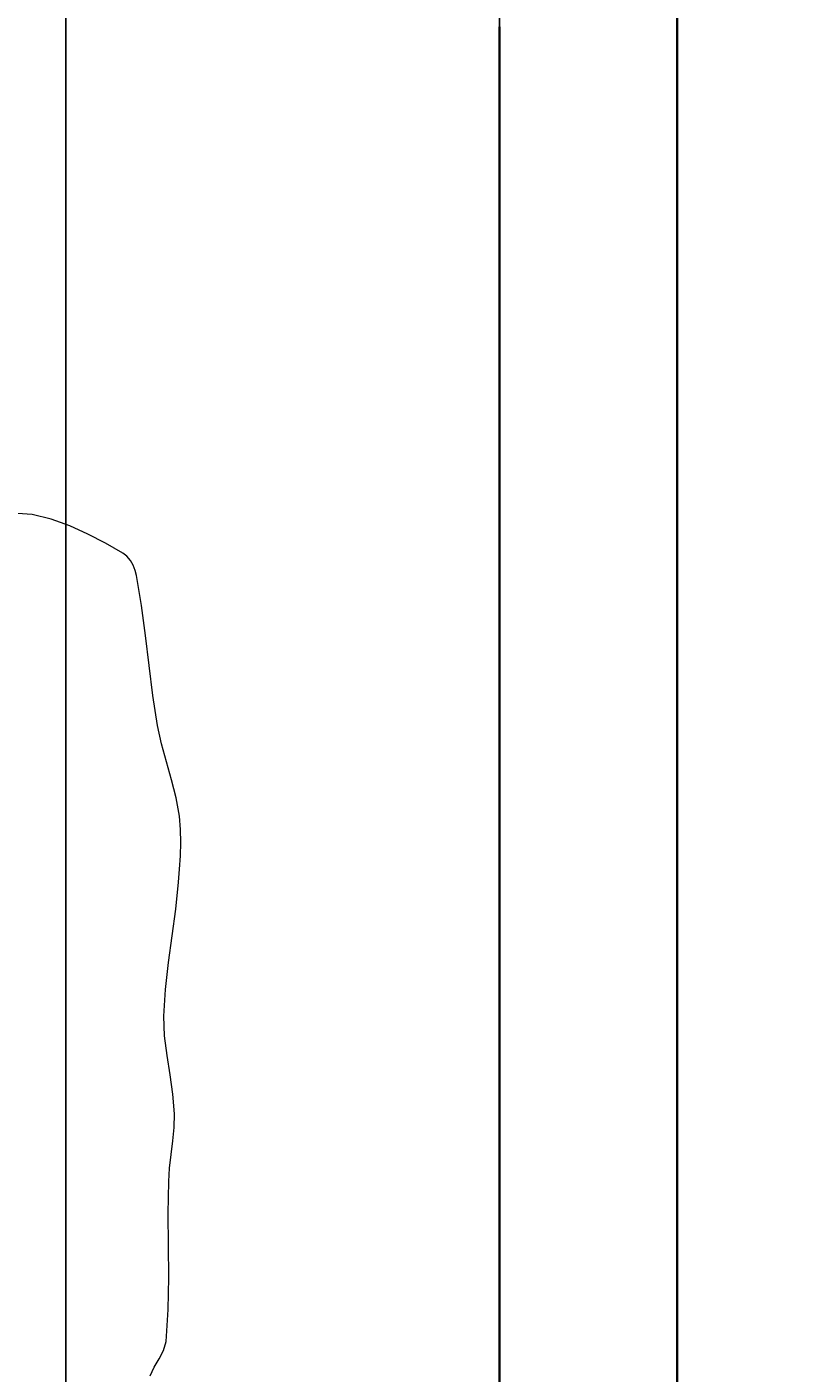
# Model space of a CAD drawing. Units: inches. Extents: x 1770 to 2988, y 1161 to 3221.
# Tile 29 of 44: x 2593 to 2631, y 2300 to 2368. Entities that reach past the tile are written whole.
import ezdxf

# ---------------------------------------------------------------- set-up
doc = ezdxf.new("R2010")
doc.units = ezdxf.units.IN
for name, color, linetype, lineweight in [('A-ANNO-DIMS', 2, 'Continuous', 18), ('A-FURN', 8, 'Continuous', 13), ('A-WALL', 7, 'Continuous', 35)]:
    doc.layers.add(name, color=color, linetype=linetype, lineweight=lineweight)
doc.styles.get("Standard").update_dxf_attribs({"font": 'arial.ttf'})
doc.dimstyles.get("Standard").update_dxf_attribs({"dimtxt": 0.18, "dimasz": 0.18, "dimexe": 0.18, "dimexo": 0.0625, "dimgap": 0.09, "dimtad": 0, "dimtih": 1, "dimtoh": 1, "dimdec": 4, "dimzin": 0, "dimdsep": 46, "dimtxsty": 'Standard', "dimcen": 0.09, "dimadec": 0, "dimazin": 0, "dimtfac": 1, "dimtdec": 4, "dimtofl": 0, "dimtmove": 0, "dimatfit": 3, "dimfxl": 1, "dimtolj": 1, "dimtzin": 0, "dimarcsym": 0})

# ---------------------------------------------------------------- blocks, each defined once
blk = doc.blocks.new('BED-DOUBLE-PLAN')
for p, q in [((67.458, 87.108), (66.715, 87.159)), ((68.424, 86.867), (67.458, 87.108)), ((69.364, 86.53), (68.424, 86.867)), ((70.28, 86.118), (69.364, 86.53)), ((71.172, 85.653), (70.28, 86.118)), ((72.043, 85.157), (71.172, 85.653)), ((72.253, 84.994), (72.043, 85.157)), ((72.425, 84.785), (72.253, 84.994)), ((72.561, 84.542), (72.425, 84.785)), ((72.662, 84.282), (72.561, 84.542)), ((72.731, 84.019), (72.662, 84.282)), ((72.993, 82.51), (72.731, 84.019)), ((73.197, 80.991), (72.993, 82.51)), ((73.377, 79.468), (73.197, 80.991)), ((73.567, 77.947), (73.377, 79.468)), ((73.802, 76.433), (73.567, 77.947)), ((74.003, 75.51), (73.802, 76.433)), ((74.25, 74.596), (74.003, 75.51)), ((74.506, 73.685), (74.25, 74.596)), ((74.736, 72.768), (74.506, 73.685)), ((74.904, 71.84), (74.736, 72.768)), ((74.965, 71.175), (74.904, 71.84)), ((74.978, 70.506), (74.965, 71.175)), ((74.957, 69.836), (74.978, 70.506)), ((74.914, 69.165), (74.957, 69.836)), ((74.862, 68.497), (74.914, 69.165)), ((74.721, 67.139), (74.862, 68.497)), ((74.536, 65.785), (74.721, 67.139)), ((74.348, 64.431), (74.536, 65.785)), ((74.196, 63.075), (74.348, 64.431)), ((74.12, 61.714), (74.196, 63.075)), ((74.159, 60.723), (74.12, 61.714)), ((74.28, 59.737), (74.159, 60.723)), ((74.435, 58.752), (74.28, 59.737)), ((74.575, 57.766), (74.435, 58.752)), ((74.652, 56.776), (74.575, 57.766)), ((74.639, 56.089), (74.652, 56.776)), ((74.578, 55.403), (74.639, 56.089)), ((74.494, 54.718), (74.578, 55.403)), ((74.414, 54.032), (74.494, 54.718)), ((74.365, 53.345), (74.414, 54.032)), ((74.338, 51.727), (74.365, 53.345)), ((74.351, 50.106), (74.338, 51.727)), ((74.364, 48.487), (74.351, 50.106)), ((74.337, 46.869), (74.364, 48.487)), ((74.232, 45.256), (74.337, 46.869)), ((74.11, 44.804), (74.232, 45.256)), ((73.637, 43.953), (73.887, 44.375)), ((73.887, 44.375), (74.11, 44.804)), ((73.435, 43.523), (73.637, 43.953))]:
    blk.add_line(p, q)
blk = doc.blocks.new('*D61')
at = {"layer": 'A-ANNO-DIMS', "color": 0, "lineweight": -2, "transparency": 16777216}
for p, q in [((2625.758, 2376.702), (2866.867, 2376.702)), ((2866.687, 2376.522), (2866.687, 1993.634)), ((2866.687, 1610.382), (2866.687, 1993.27)), ((2625.758, 1610.202), (2866.867, 1610.202))]:
    blk.add_line(p, q, dxfattribs=at)
at = {"layer": 'A-ANNO-DIMS', "color": 0, "transparency": 16777216}
for points in [[(2866.657, 2376.522), (2866.717, 2376.522), (2866.687, 2376.702)], [(2866.657, 1610.382), (2866.717, 1610.382), (2866.687, 1610.202)]]:
    blk.add_solid(points, dxfattribs=at)
at = {"layer": 'Defpoints', "color": 0, "transparency": 16777216}
for p in [(2625.696, 2376.702), (2866.687, 2376.702), (2625.696, 1610.202)]:
    blk.add_point(p, dxfattribs=at)
at = {"layer": 'A-ANNO-DIMS', "color": 0, "transparency": 16777216, "insert": (2866.687, 1993.452), "char_height": 0.18, "attachment_point": 5}
blk.add_mtext('\\A1;766.5', dxfattribs=at)
blk = doc.blocks.new('*D84')
at = {"layer": 'A-ANNO-DIMS', "color": 0, "lineweight": -2, "transparency": 16777216}
for p, q in [((2513.196, 1835.265), (2513.196, 2570.705)), ((2513.376, 2570.525), (2564.56, 2570.525)), ((2616.516, 2570.525), (2565.332, 2570.525)), ((2616.696, 1835.265), (2616.696, 2570.705))]:
    blk.add_line(p, q, dxfattribs=at)
at = {"layer": 'A-ANNO-DIMS', "color": 0, "transparency": 16777216}
for points in [[(2513.376, 2570.555), (2513.376, 2570.495), (2513.196, 2570.525)], [(2616.516, 2570.555), (2616.516, 2570.495), (2616.696, 2570.525)]]:
    blk.add_solid(points, dxfattribs=at)
at = {"layer": 'Defpoints', "color": 0, "transparency": 16777216}
for p in [(2616.696, 2570.525), (2513.196, 1835.202), (2616.696, 1835.202)]:
    blk.add_point(p, dxfattribs=at)
at = {"layer": 'A-ANNO-DIMS', "color": 0, "transparency": 16777216, "insert": (2564.946, 2570.525), "char_height": 0.18, "attachment_point": 5}
blk.add_mtext('\\A1;103.5', dxfattribs=at)
blk = doc.blocks.new('*D86')
at = {"layer": 'A-ANNO-DIMS', "color": 0, "lineweight": -2, "transparency": 16777216}
for p, q in [((2583.196, 1775.211), (2583.196, 2570.705)), ((2583.376, 2570.525), (2599.622, 2570.525)), ((2616.516, 2570.525), (2600.27, 2570.525)), ((2616.696, 1775.265), (2616.696, 2570.705))]:
    blk.add_line(p, q, dxfattribs=at)
at = {"layer": 'A-ANNO-DIMS', "color": 0, "transparency": 16777216}
for points in [[(2583.376, 2570.555), (2583.376, 2570.495), (2583.196, 2570.525)], [(2616.516, 2570.555), (2616.516, 2570.495), (2616.696, 2570.525)]]:
    blk.add_solid(points, dxfattribs=at)
at = {"layer": 'Defpoints', "color": 0, "transparency": 16777216}
for p in [(2616.696, 2570.525), (2583.196, 1775.149), (2616.696, 1775.202)]:
    blk.add_point(p, dxfattribs=at)
at = {"layer": 'A-ANNO-DIMS', "color": 0, "transparency": 16777216, "insert": (2599.946, 2570.525), "char_height": 0.18, "attachment_point": 5}
blk.add_mtext('\\A1;33.5', dxfattribs=at)
blk = doc.blocks.new('*D87')
at = {"layer": 'A-ANNO-DIMS', "color": 0, "lineweight": -2, "transparency": 16777216}
for p, q in [((2594.748, 1861.402), (2594.748, 2570.705)), ((2594.928, 2570.525), (2605.326, 2570.525)), ((2616.516, 2570.525), (2606.118, 2570.525)), ((2616.696, 1839.765), (2616.696, 2570.705))]:
    blk.add_line(p, q, dxfattribs=at)
at = {"layer": 'A-ANNO-DIMS', "color": 0, "transparency": 16777216}
for points in [[(2594.928, 2570.555), (2594.928, 2570.495), (2594.748, 2570.525)], [(2616.516, 2570.555), (2616.516, 2570.495), (2616.696, 2570.525)]]:
    blk.add_solid(points, dxfattribs=at)
at = {"layer": 'Defpoints', "color": 0, "transparency": 16777216}
for p in [(2616.696, 2570.525), (2594.748, 1861.34), (2616.696, 1839.702)]:
    blk.add_point(p, dxfattribs=at)
at = {"layer": 'A-ANNO-DIMS', "color": 0, "transparency": 16777216, "insert": (2605.722, 2570.525), "char_height": 0.18, "attachment_point": 5}
blk.add_mtext('\\A1;21.95', dxfattribs=at)

msp = doc.modelspace()

# ---------------------------------------------------------------- linework, layer by layer
at = {"layer": 'A-WALL'}
for p, q in [((2625.696, 2376.7021), (2625.696, 1610.2021)), ((2616.696, 2367.7021), (2616.696, 2175.7021))]:
    msp.add_line(p, q, dxfattribs=at)

# ---------------------------------------------------------------- block references
at = {"layer": 'A-FURN'}
msp.add_blockref('BED-DOUBLE-PLAN', (2525.5949, 2255.9126), dxfattribs=at)

# ---------------------------------------------------------------- dimensions: what is measured, and where the dimension line sits
at = {"layer": 'A-ANNO-DIMS'}
for p1, p2, override, picture, middle in [((2513.196, 1835.2021), (2616.696, 1835.2021), {"dimdec": 1, "dimlfac": 1, "dimrnd": 0, "dimzin": 0, "dimdsep": 46, "dimlunit": 2}, '*D84', (2564.946, 2570.5247)), ((2583.196, 1775.149), (2616.696, 1775.2021), {"dimdec": 1, "dimlfac": 1, "dimrnd": 0, "dimzin": 0, "dimdsep": 46, "dimlunit": 2}, '*D86', (2599.946, 2570.5247)), ((2594.7479, 1861.3395), (2616.696, 1839.7021), {"dimdec": 2, "dimlfac": 1, "dimrnd": 0, "dimzin": 0, "dimdsep": 46, "dimlunit": 2}, '*D87', (2605.7219, 2570.5247))]:
    dim = msp.add_linear_dim(base=(2616.696, 2570.5247), p1=p1, p2=p2, dimstyle='Standard', override=override, dxfattribs=at)
    dim.commit()
    dim.dimension.update_dxf_attribs({"geometry": picture, "text_midpoint": middle})
dim = msp.add_linear_dim(base=(2866.6874, 2376.7021), p1=(2625.696, 1610.2021), p2=(2625.696, 2376.7021), angle=90, dimstyle='Standard', override={"dimdec": 1, "dimlfac": 1, "dimrnd": 0, "dimzin": 0, "dimdsep": 46, "dimlunit": 2}, dxfattribs=at)
dim.commit()
dim.dimension.update_dxf_attribs({"geometry": '*D61', "text_midpoint": (2866.6874, 1993.4521)})

doc.saveas('drawing.dxf')
